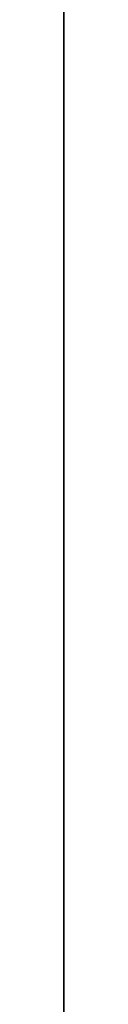
# Model space of a CAD drawing. Units: inches. Extents: x 2083 to 3317, y 1141 to 2115.
# Tile 44 of 256: x 2235.9598 to 2235.9598, y 1478.1958 to 1478.7355. Entities that reach past the tile are written whole.
import ezdxf

# ---------------------------------------------------------------- set-up
doc = ezdxf.new("R2010")
doc.units = ezdxf.units.IN
doc.layers.add('A-ANNO-DIMS', color=2, linetype='Continuous', lineweight=18)
doc.layers.add('A-WALL', color=7, linetype='Continuous', lineweight=35)
doc.layers.add('A-WALL-PATT', color=251, linetype='Continuous', lineweight=13, true_color=0x636466)
doc.styles.get("Standard").update_dxf_attribs({"font": 'arial.ttf'})
doc.dimstyles.new('ISO-25', dxfattribs={"dimtxt": 12, "dimasz": 12, "dimexe": 1.25, "dimexo": 0.625, "dimtad": 1, "dimlunit": 3, "dimtxsty": 'Standard', "dimcen": 2.5, "dimadec": 0, "dimazin": 0, "dimtfac": 1, "dimtmove": 0, "dimatfit": 3, "dimfxl": 1, "dimarcsym": 0})

# ---------------------------------------------------------------- blocks, each defined once
blk = doc.blocks.new('*D30')
at = {"layer": 'A-ANNO-DIMS', "color": 0, "lineweight": -2, "transparency": 16777216}
for p, q in [((2240.01786, 1445.27381), (2240.01786, 1448.04553)), ((2254.32933, 1445.27381), (2254.32933, 1448.04553)), ((2228.01786, 1446.79553), (2216.01786, 1446.79553)), ((2240.01786, 1446.79553), (2254.32933, 1446.79553)), ((2266.32933, 1446.79553), (2413.76487, 1446.79553))]:
    blk.add_line(p, q, dxfattribs=at)
at = {"layer": 'A-ANNO-DIMS', "color": 0, "transparency": 16777216}
for points in [[(2228.01786, 1448.79553), (2228.01786, 1444.79553), (2240.01786, 1446.79553)], [(2266.32933, 1448.79553), (2266.32933, 1444.79553), (2254.32933, 1446.79553)]]:
    blk.add_solid(points, dxfattribs=at)
at = {"layer": 'Defpoints', "color": 0, "transparency": 16777216}
for p in [(2254.32933, 1446.79553), (2240.01786, 1444.64881), (2254.32933, 1444.64881)]:
    blk.add_point(p, dxfattribs=at)
at = {"layer": 'A-ANNO-DIMS', "color": 0, "transparency": 16777216, "insert": (2346.0471, 1453.62517), "char_height": 12, "attachment_point": 5}
blk.add_mtext('WC 1\'-2 1/2" TYP.', dxfattribs=at)
blk = doc.blocks.new('*D31')
at = {"layer": 'A-ANNO-DIMS', "color": 0, "lineweight": -2, "transparency": 16777216}
for p, q in [((2237.87114, 1456.64881), (2237.87114, 1541.91518)), ((2239.39286, 1444.64881), (2236.62114, 1444.64881)), ((2237.87114, 1431.54754), (2237.87114, 1444.64881)), ((2239.39286, 1431.54754), (2236.62114, 1431.54754)), ((2237.87114, 1419.54754), (2237.87114, 1407.54754))]:
    blk.add_line(p, q, dxfattribs=at)
at = {"layer": 'A-ANNO-DIMS', "color": 0, "transparency": 16777216}
for points in [[(2235.87114, 1456.64881), (2239.87114, 1456.64881), (2237.87114, 1444.64881)], [(2235.87114, 1419.54754), (2239.87114, 1419.54754), (2237.87114, 1431.54754)]]:
    blk.add_solid(points, dxfattribs=at)
at = {"layer": 'Defpoints', "color": 0, "transparency": 16777216}
for p in [(2237.87114, 1444.64881), (2240.01786, 1444.64881), (2240.01786, 1431.54754)]:
    blk.add_point(p, dxfattribs=at)
at = {"layer": 'A-ANNO-DIMS', "color": 0, "transparency": 16777216, "insert": (2231.21749, 1505.28199), "char_height": 12, "attachment_point": 5, "rotation": 90}
blk.add_mtext('1\'-1" TYP.', dxfattribs=at)
blk = doc.blocks.new('*D45')
at = {"layer": 'A-ANNO-DIMS', "color": 0, "lineweight": -2, "transparency": 16777216}
for p, q in [((2235.95978, 1478.38636), (2235.95978, 1531.36136)), ((2418.95978, 1478.38636), (2418.95978, 1531.36136)), ((2247.95978, 1530.11136), (2406.95978, 1530.11136))]:
    blk.add_line(p, q, dxfattribs=at)
at = {"layer": 'A-ANNO-DIMS', "color": 0, "transparency": 16777216}
for points in [[(2247.95978, 1532.11136), (2247.95978, 1528.11136), (2235.95978, 1530.11136)], [(2406.95978, 1532.11136), (2406.95978, 1528.11136), (2418.95978, 1530.11136)]]:
    blk.add_solid(points, dxfattribs=at)
at = {"layer": 'Defpoints', "color": 0, "transparency": 16777216}
for p in [(2418.95978, 1530.11136), (2235.95978, 1477.76136), (2418.95978, 1477.76136)]:
    blk.add_point(p, dxfattribs=at)
at = {"layer": 'A-ANNO-DIMS', "color": 0, "transparency": 16777216, "insert": (2327.45978, 1536.86733), "char_height": 12, "attachment_point": 5}
blk.add_mtext('15\'-3"', dxfattribs=at)
blk = doc.blocks.new('*D62')
at = {"layer": 'A-ANNO-DIMS', "color": 0, "lineweight": -2, "transparency": 16777216}
for p, q in [((2235.95978, 1469.38636), (2235.95978, 1522.36136)), ((2379.95978, 1469.38636), (2379.95978, 1522.36136)), ((2247.95978, 1521.11136), (2367.95978, 1521.11136))]:
    blk.add_line(p, q, dxfattribs=at)
at = {"layer": 'A-ANNO-DIMS', "color": 0, "transparency": 16777216}
for points in [[(2247.95978, 1523.11136), (2247.95978, 1519.11136), (2235.95978, 1521.11136)], [(2367.95978, 1523.11136), (2367.95978, 1519.11136), (2379.95978, 1521.11136)]]:
    blk.add_solid(points, dxfattribs=at)
at = {"layer": 'Defpoints', "color": 0, "transparency": 16777216}
for p in [(2379.95978, 1521.11136), (2235.95978, 1468.76136), (2379.95978, 1468.76136)]:
    blk.add_point(p, dxfattribs=at)
at = {"layer": 'A-ANNO-DIMS', "color": 0, "transparency": 16777216, "insert": (2307.95978, 1527.86324), "char_height": 12, "attachment_point": 5}
blk.add_mtext('12\'-0"', dxfattribs=at)

msp = doc.modelspace()

# ---------------------------------------------------------------- hatches: boundary and pattern name
at = {"layer": 'A-WALL-PATT'}
h = msp.add_hatch(color=256, dxfattribs=at)
h.dxf.hatch_style = 1
h.paths.add_polyline_path([(3126.95978, 2020.76136), (2748.95978, 2020.76136), (2604.95978, 2020.76136), (2226.95978, 2020.76136), (2226.95978, 1702.76136), (2466.95978, 1702.76136), (2466.95978, 1582.76136), (2418.95978, 1582.76136), (2418.95978, 1477.76136), (2226.95978, 1477.76136), (2226.95978, 1263.26136), (2544.95978, 1263.26136), (2544.95978, 1411.76136), (2604.95978, 1411.76136), (2685.95978, 1411.76136), (2685.95978, 1420.76136), (2604.95978, 1420.76136), (2604.95978, 1573.76136), (2604.95978, 1702.76136), (2604.95978, 2011.76136), (2748.95978, 2011.76136), (2748.95978, 1702.76136), (2862.95978, 1702.76136), (2862.95978, 1621.76136), (2871.95978, 1621.76136), (2871.95978, 1702.76136), (2883.95978, 1702.76136), (2883.95978, 1706.93946, -0.026459), (2883.95978, 1711.76136), (2757.95978, 1711.76136), (2757.95978, 1807.76136), (2787.95978, 1807.76136), (2787.95978, 1812.26136), (2757.95978, 1812.26136), (2757.95978, 2011.76136), (2877.95978, 2011.76136), (2877.95978, 1812.26136), (2847.95978, 1812.26136), (2847.95978, 1807.76136), (2889.83574, 1807.76136), (2889.83574, 1812.26136), (2882.45978, 1812.26136), (2882.45978, 2011.76136), (3117.95978, 2011.76136), (3117.95978, 1812.26136), (2937.83574, 1812.26136), (2937.83574, 1807.76136), (2995.70978, 1807.76136), (2995.70978, 1796.11767), (3000.20978, 1796.11767), (3000.20978, 1807.76136), (3117.95978, 1807.76136), (3117.95978, 1711.76136), (3000.20978, 1711.76136), (3000.20978, 1760.11767), (2998.5727, 1760.11767, -0.020711), (2995.70978, 1760.11767), (2995.70978, 1711.76136), (2931.95978, 1711.76136), (2931.95978, 1702.76136), (3126.95978, 1702.76136)])
h.paths.add_polyline_path([(2471.45978, 2011.76136), (2471.45978, 1810.01136), (2462.71694, 1810.01136), (2462.71694, 1805.51136), (2505.95978, 1805.51136), (2505.95978, 1810.01136), (2475.95978, 1810.01136), (2475.95978, 2011.76136), (2595.95978, 2011.76136), (2595.95978, 1810.01136), (2565.95978, 1810.01136), (2565.95978, 1805.51136), (2595.95978, 1805.51136), (2595.95978, 1711.76136), (2235.95978, 1711.76136), (2235.95978, 1805.51136), (2353.70978, 1805.51136), (2353.70978, 1796.05416), (2358.20978, 1796.05416), (2358.20978, 1805.51136), (2414.71694, 1805.51136), (2414.71694, 1810.01136), (2235.95978, 1810.01136), (2235.95978, 2011.76136)], flags=16)
h.paths.add_polyline_path([(2270.20473, 1994.61001), (2270.20473, 1970.61001), (2246.20473, 1970.61001), (2246.20473, 1994.61001)], flags=0)
edge = h.paths.add_edge_path(flags=0)
edge.add_ellipse((2332.02739, 1899.79818), major_axis=(-3.04299, 3.04299), ratio=0.1682525, start_angle=-161.33217, end_angle=-156.30711, ccw=False)
edge.add_ellipse((2333.08204, 1898.74353), major_axis=(-1.05465, 1.05465), ratio=0.4535321, start_angle=-123.37102, end_angle=-94.15911)
edge = h.paths.add_edge_path(flags=0)
edge.add_ellipse((2332.02739, 1968.87629), major_axis=(3.04299, 3.04299), ratio=0.1682525, start_angle=18.66783, end_angle=23.69289)
edge.add_spline(control_points=[(2332.9256, 1970.6911), (2332.22677, 1970.3361), (2330.89371, 1969.65891), (2328.41308, 1970.93214), (2327.20393, 1967.74871), (2324.7096, 1969.95559), (2322.53282, 1967.01235), (2320.01285, 1971.29581), (2317.68031, 1968.15784), (2316.04053, 1967.10205), (2315.4269, 1966.8096)], knot_values=[0, 0, 0, 0, 2.267059, 4.324559, 6.685584, 8.878641, 11.121502, 14.300359, 17.755284, 19.732645, 19.732645, 19.732645, 19.732645], degree=3, periodic=0)
edge.add_ellipse((2332.02739, 1968.87629), major_axis=(3.04299, 3.04299), ratio=0.1682525, start_angle=18.66783, end_angle=23.69289, ccw=False)
edge.add_ellipse((2333.08204, 1969.93094), major_axis=(1.05465, 1.05465), ratio=0.4535321, start_angle=56.62898, end_angle=85.84089, ccw=False)
edge = h.paths.add_edge_path(flags=0)
edge.add_spline(control_points=[(2296.42829, 1967.98791), (2293.6278, 1965.33631), (2287.70362, 1959.72709), (2299.74386, 1949.9957), (2294.53259, 1935.66853), (2290.57323, 1920.60351), (2293.39412, 1909.97369), (2296.18541, 1904.96654)], knot_values=[0.099185, 0.099185, 0.099185, 0.099185, 0.345301, 0.619822, 0.982653, 1.386093, 1.810555, 1.810555, 1.810555, 1.810555], degree=3, periodic=0)
edge.add_spline(control_points=[(2296.18541, 1904.96654), (2297.38358, 1902.6193), (2298.00097, 1901.94931), (2298.55297, 1901.46815)], knot_values=[0.006246, 0.006246, 0.006246, 0.006246, 0.055476, 0.055476, 0.055476, 0.055476], degree=3, periodic=0)
edge.add_spline(control_points=[(2298.55297, 1901.46815), (2297.25861, 1900.92322), (2295.22529, 1900.23213), (2293.06023, 1900.61421), (2292.10142, 1900.78841), (2292.08958, 1900.79057)], knot_values=[0.312835, 0.312835, 0.312835, 0.312835, 0.40178, 0.474987, 0.475903, 0.475903, 0.475903, 0.475903], degree=3, periodic=0)
edge.add_arc((2292.79365, 1904.66411), 3.93701, 215.4209, 259.69818, ccw=False)
edge.add_spline(control_points=[(2289.58531, 1902.3823), (2289.47665, 1902.53509), (2289.36848, 1902.68804), (2289.26086, 1902.84117)], knot_values=[0.102872, 0.102872, 0.102872, 0.102872, 0.116896, 0.116896, 0.116896, 0.116896], degree=3, periodic=0)
edge.add_spline(control_points=[(2289.26086, 1902.84117), (2288.6866, 1902.55019), (2287.64005, 1902.0199), (2285.88134, 1901.87395), (2283.85297, 1901.50435), (2281.71999, 1899.71054), (2278.46699, 1899.49294), (2276.15714, 1901.8832), (2272.25895, 1899.80407), (2267.77761, 1901.84318), (2262.24388, 1900.18403), (2257.41493, 1901.78206), (2254.31837, 1900.72612), (2253.17828, 1900.33734)], knot_values=[0, 0, 0, 0, 1.907977, 3.477176, 5.261074, 7.972851, 11.680248, 13.717921, 16.939592, 22.789562, 27.502503, 33.595215, 37.145618, 37.145618, 37.145618, 37.145618], degree=3, periodic=0)
edge.add_line((2253.17828, 1900.33734), (2250.24424, 1902.84117))
edge.add_line((2250.24424, 1902.84117), (2250.24424, 1965.8333))
edge.add_line((2250.24424, 1965.8333), (2253.17828, 1968.33712))
edge.add_spline(control_points=[(2253.17828, 1968.33712), (2254.31837, 1967.94835), (2257.41493, 1966.89241), (2262.24388, 1968.49043), (2267.77761, 1966.83128), (2271.52673, 1968.53722), (2273.87591, 1967.82829), (2274.2067, 1967.72764)], knot_values=[0, 0, 0, 0, 0.09018, 0.244935, 0.364644, 0.513233, 0.537855, 0.537855, 0.537855, 0.537855], degree=3, periodic=0)
edge.add_arc((2274.35289, 1963.79335), 3.93701, 72.05113, 92.12795, ccw=False)
edge.add_arc((2281.29693, 1985.23), 18.5963, 252.051134, 288.565722)
edge.add_arc((2292.31672, 1956.02888), 12.64608, 71.026788, 113.778218, ccw=False)
edge = h.paths.add_edge_path(flags=0)
edge.add_spline(control_points=[(2274.89941, 1951.85619), (2275.06616, 1951.61659), (2275.23269, 1951.37659), (2275.39799, 1951.13585)], knot_values=[1.409916, 1.409916, 1.409916, 1.409916, 1.43159, 1.43159, 1.43159, 1.43159], degree=3, periodic=0)
edge.add_spline(control_points=[(2275.39799, 1951.13585), (2275.79211, 1950.56189), (2276.17923, 1949.98377), (2276.54555, 1949.3971)], knot_values=[1.358238, 1.358238, 1.358238, 1.358238, 1.409916, 1.409916, 1.409916, 1.409916], degree=3, periodic=0)
edge.add_line((2276.54555, 1949.3971), (2277.43729, 1947.86218))
edge.add_spline(control_points=[(2277.43729, 1947.86218), (2276.30383, 1945.67311), (2274.6397, 1942.42688), (2274.63161, 1938.0939), (2272.79912, 1930.85155), (2274.35643, 1943.89705), (2275.94768, 1947.92336), (2276.54555, 1949.3971)], knot_values=[0.005632, 0.005632, 0.005632, 0.005632, 0.186014, 0.266002, 0.357087, 0.59639, 0.739732, 0.739732, 0.739732, 0.739732], degree=3, periodic=0)
edge.add_spline(control_points=[(2276.54555, 1949.3971), (2276.17923, 1949.98377), (2275.79211, 1950.56189), (2275.39799, 1951.13585)], knot_values=[1.358238, 1.358238, 1.358238, 1.358238, 1.409916, 1.409916, 1.409916, 1.409916], degree=3, periodic=0)
edge.add_spline(control_points=[(2275.39799, 1951.13585), (2274.9425, 1950.08045), (2274.20776, 1948.02527), (2273.9346, 1944.85148), (2272.46853, 1937.62749), (2273.46622, 1945.69647), (2274.70062, 1951.05947), (2274.89941, 1951.85619)], knot_values=[0.104364, 0.104364, 0.104364, 0.104364, 0.189636, 0.269624, 0.36071, 0.600013, 0.644622, 0.644622, 0.644622, 0.644622], degree=3, periodic=0)
h.paths.add_polyline_path([(2269.16751, 1963.12757, -0.357527), (2268.17063, 1960.97637, -0.092561), (2268.17063, 1939.43632, -0.357527), (2269.16751, 1937.28512, -0.357527), (2267.01631, 1938.282, -0.164785), (2254.68558, 1938.282, -0.357527), (2252.53438, 1937.28512, -0.357527), (2253.53126, 1939.43632, -0.092561), (2253.53126, 1960.97637, -0.357527), (2252.53438, 1963.12757, -0.357527), (2254.68558, 1962.13069, -0.164785), (2267.01631, 1962.13069, -0.357527)], flags=0)
h.paths.add_polyline_path([(2248.87407, 1967.8018), (2248.87407, 1957.02771), (2249.45778, 1957.02771), (2249.45778, 1911.64676), (2248.87407, 1911.64676), (2248.87407, 1900.87267), (2246.51186, 1900.87267, 0.197327), (2244.14966, 1902.45687), (2244.14966, 1966.21759, 0.197327), (2246.51186, 1967.8018)], flags=0)
h.paths.add_polyline_path([(2269.16751, 1931.38934, -0.357527), (2268.17063, 1929.23814, -0.092561), (2268.17063, 1907.6981, -0.357527), (2269.16751, 1905.54689, -0.357527), (2267.01631, 1906.54377, -0.164785), (2254.68558, 1906.54377, -0.357527), (2252.53438, 1905.54689, -0.357527), (2253.53126, 1907.6981, -0.092561), (2253.53126, 1929.23814, -0.357527), (2252.53438, 1931.38934, -0.357527), (2254.68558, 1930.39246, -0.164785), (2267.01631, 1930.39246, -0.357527)], flags=0)
edge = h.paths.add_edge_path(flags=0)
edge.add_spline(control_points=[(2276.19686, 1906.7237), (2276.16814, 1909.02893), (2276.11405, 1913.37185), (2270.59842, 1924.92498), (2273.90517, 1919.01278), (2275.92171, 1916.26206), (2275.47457, 1912.40215), (2277.25787, 1910.38062), (2276.69604, 1908.22504), (2276.64622, 1906.81302), (2276.61782, 1906.00841)], knot_values=[0, 0, 0, 0, 8.61026, 16.221274, 18.843057, 23.804898, 27.440828, 29.356102, 31.203478, 33.650687, 33.650687, 33.650687, 33.650687], degree=3, periodic=0)
edge.add_spline(control_points=[(2276.61782, 1906.00841), (2276.62331, 1905.62414), (2276.49774, 1904.62866), (2275.44178, 1903.85473), (2274.93731, 1903.08045), (2274.85908, 1902.84117)], knot_values=[0.156488, 0.156488, 0.156488, 0.156488, 0.184398, 0.231376, 0.250598, 0.250598, 0.250598, 0.250598], degree=3, periodic=0)
edge.add_line((2274.85908, 1902.84117), (2276.50598, 1902.84117))
edge.add_spline(control_points=[(2276.50598, 1902.84117), (2276.78831, 1903.08494), (2277.66507, 1904.1252), (2278.24954, 1904.34074), (2277.65387, 1908.52739), (2278.15567, 1906.22781), (2278.10046, 1905.28595), (2278.84667, 1904.06901), (2277.85679, 1903.41495), (2277.87419, 1902.99105), (2277.90356, 1902.84117)], knot_values=[0.059574, 0.059574, 0.059574, 0.059574, 0.080753, 0.103741, 0.16972, 0.176036, 0.207137, 0.240474, 0.262341, 0.27366, 0.27366, 0.27366, 0.27366], degree=3, periodic=0)
edge.add_line((2277.90356, 1902.84117), (2280.02983, 1902.84117))
edge.add_spline(control_points=[(2280.02983, 1902.84117), (2279.88822, 1903.0884), (2279.49926, 1903.98155), (2280.15228, 1905.93935), (2278.10362, 1909.65776), (2279.76239, 1907.18529), (2280.3279, 1904.87486), (2280.48511, 1903.48959), (2281.46327, 1903.24943), (2281.75834, 1902.9365), (2281.83404, 1902.84117)], knot_values=[0.013856, 0.013856, 0.013856, 0.013856, 0.034874, 0.088867, 0.107879, 0.126738, 0.158714, 0.193757, 0.217487, 0.226722, 0.226722, 0.226722, 0.226722], degree=3, periodic=0)
edge.add_spline(control_points=[(2281.83404, 1902.84117), (2281.78753, 1902.8267), (2281.64702, 1902.78299), (2281.39553, 1902.85949), (2281.08808, 1902.98524), (2280.72068, 1903.0609), (2280.33345, 1903.02573), (2280.12477, 1902.89888), (2280.02983, 1902.84117)], knot_values=[0, 0, 0, 0, 0.14413, 0.435517, 0.749276, 1.153046, 1.548371, 1.878348, 1.878348, 1.878348, 1.878348], degree=3, periodic=0)
edge.add_line((2280.02983, 1902.84117), (2277.90356, 1902.84117))
edge.add_spline(control_points=[(2277.90356, 1902.84117), (2277.89286, 1902.79586), (2277.8654, 1902.67964), (2277.60748, 1902.68748), (2277.27405, 1902.8007), (2276.83792, 1902.61977), (2276.58381, 1902.78926), (2276.50598, 1902.84117)], knot_values=[0, 0, 0, 0, 0.127189, 0.326199, 0.628009, 1.24357, 1.515331, 1.515331, 1.515331, 1.515331], degree=3, periodic=0)
edge.add_line((2276.50598, 1902.84117), (2274.85908, 1902.84117))
edge.add_spline(control_points=[(2274.85908, 1902.84117), (2274.81444, 1902.89859), (2274.72513, 1903.01345), (2274.49348, 1903.11897), (2274.24429, 1902.96054), (2273.93712, 1903.18494), (2273.61404, 1902.98314), (2273.40832, 1902.88304), (2273.32225, 1902.84117)], knot_values=[0, 0, 0, 0, 0.21843, 0.436957, 0.687977, 0.990379, 1.398396, 1.69185, 1.69185, 1.69185, 1.69185], degree=3, periodic=0)
edge.add_spline(control_points=[(2273.32225, 1902.84117), (2273.61674, 1903.44569), (2274.274, 1904.53825), (2276.02724, 1904.5737), (2276.20696, 1906.58364), (2276.19686, 1906.7237)], knot_values=[0.012227, 0.012227, 0.012227, 0.012227, 0.059472, 0.106218, 0.134458, 0.134458, 0.134458, 0.134458], degree=3, periodic=0)
h.paths.add_polyline_path([(2270.77605, 1897.78983), (2270.77605, 1873.78983), (2246.77605, 1873.78983), (2246.77605, 1897.78983)], flags=0)
h.paths.add_polyline_path([(2353.70978, 1760.00506), (2353.70978, 1760.05416), (2358.20978, 1760.05416, -0.033729)], flags=0)
h.paths.add_polyline_path([(2321.81912, 1737.52919), (2341.99533, 1737.52919, -0.414214), (2343.20327, 1736.32124), (2343.20327, 1721.0206, -0.414214), (2341.99533, 1719.81265), (2321.81912, 1719.81265, -0.414214), (2320.61117, 1721.0206), (2320.61117, 1736.32124, -0.414214)], flags=0)
h.paths.add_polyline_path([(2324.23501, 1736.32124), (2339.57944, 1736.32124, -0.414214), (2341.99533, 1733.90535), (2341.99533, 1725.44973, -0.414214), (2339.57944, 1723.03384), (2333.68059, 1723.03384), (2333.84532, 1722.04547, -0.870646), (2335.4254, 1721.82589, -0.767327), (2333.92269, 1721.42324), (2331.29102, 1721.42324, -0.767327), (2329.78832, 1721.82589, -0.870646), (2331.3684, 1722.04547), (2331.53313, 1723.03384), (2324.23501, 1723.03384, -0.414214), (2321.81912, 1725.44973), (2321.81912, 1733.90535, -0.414214)], flags=0)
h.paths.add_polyline_path([(2570.48379, 1928.61544), (2589.68379, 1928.61544), (2590.16883, 1928.61544), (2590.16883, 1904.9934), (2570.48379, 1904.9934)], flags=0)
h.paths.add_polyline_path([(2574.44732, 1927.26382, -1), (2572.82884, 1927.26382, -1)], flags=0)
h.paths.add_polyline_path([(2573.08987, 1926.94088), (2573.92503, 1927.77604), (2574.14774, 1927.55333), (2573.31258, 1926.71817)], flags=0)
h.paths.add_polyline_path([(2578.77906, 1919.72962, -1), (2571.59166, 1919.72962, -1)], flags=0)
h.paths.add_polyline_path([(2578.38536, 1919.72962, -1), (2571.98536, 1919.72962, -1)], flags=0)
h.paths.add_polyline_path([(2331.59576, 1729.47622, -1), (2333.61795, 1729.47622, -1)], flags=0)
h.paths.add_polyline_path([(2578.03423, 1927.26382, -1), (2576.41574, 1927.26382, -1)], flags=0)
h.paths.add_polyline_path([(2576.68885, 1927.53109), (2576.91156, 1927.7538), (2577.74673, 1926.91863), (2577.52402, 1926.69592)], flags=0)
h.paths.add_polyline_path([(2578.13906, 1909.85954, -1), (2572.23166, 1909.85954, -1)], flags=0)
h.paths.add_polyline_path([(2577.74536, 1909.85954, -1), (2572.62536, 1909.85954, -1)], flags=0)
h.paths.add_polyline_path([(2583.79772, 1927.26382, -1), (2582.17923, 1927.26382, -1)], flags=0)
h.paths.add_polyline_path([(2582.71865, 1927.7538), (2583.55381, 1926.91863), (2583.3311, 1926.69592), (2582.49594, 1927.53109)], flags=0)
h.paths.add_polyline_path([(2582.49594, 1927.53109), (2582.71865, 1927.7538), (2583.55381, 1926.91863), (2583.3311, 1926.69592)], flags=0)
h.paths.add_polyline_path([(2587.73906, 1920.52962, -1), (2581.83166, 1920.52962, -1)], flags=0)
h.paths.add_polyline_path([(2587.34536, 1920.52962, -1), (2582.22536, 1920.52962, -1)], flags=0)
h.paths.add_polyline_path([(2587.38462, 1927.26382, -1), (2585.76613, 1927.26382, -1)], flags=0)
h.paths.add_polyline_path([(2586.08199, 1926.98025), (2586.91716, 1927.81541), (2587.13987, 1927.5927), (2586.3047, 1926.75754)], flags=0)
h.paths.add_polyline_path([(2588.37906, 1910.65954, -1), (2581.19166, 1910.65954, -1)], flags=0)
h.paths.add_polyline_path([(2587.98536, 1910.65954, -1), (2581.58536, 1910.65954, -1)], flags=0)
h.paths.add_polyline_path([(2417.16773, 1729.4779), (2437.34394, 1729.4779, -0.414214), (2438.55188, 1728.26995), (2438.55188, 1712.96931, -0.414214), (2437.34394, 1711.76136), (2417.16773, 1711.76136, -0.414214), (2415.95978, 1712.96931), (2415.95978, 1728.26995, -0.414214)], flags=0)
h.paths.add_polyline_path([(2419.58362, 1728.26995), (2434.92805, 1728.26995, -0.414214), (2437.34394, 1725.85406), (2437.34394, 1717.39844, -0.414214), (2434.92805, 1714.98255), (2429.0292, 1714.98255), (2429.19393, 1713.99418, -0.870646), (2430.77401, 1713.7746, -0.767327), (2429.2713, 1713.37195), (2426.63963, 1713.37195, -0.767327), (2425.13693, 1713.7746, -0.870646), (2426.71701, 1713.99418), (2426.88174, 1714.98255), (2419.58362, 1714.98255, -0.414214), (2417.16773, 1717.39844), (2417.16773, 1725.85406, -0.414214)], flags=0)
h.paths.add_polyline_path([(2419.58362, 1728.26995), (2434.92805, 1728.26995, -0.414214), (2437.34394, 1725.85406), (2437.34394, 1717.39844, -0.414214), (2434.92805, 1714.98255), (2429.0292, 1714.98255), (2428.35812, 1719.00903), (2427.55282, 1719.00903), (2426.88174, 1714.98255), (2419.58362, 1714.98255, -0.414214), (2417.16773, 1717.39844), (2417.16773, 1725.85406, -0.414214)], flags=0)
h.paths.add_polyline_path([(2426.94437, 1721.42492, -1), (2428.96656, 1721.42492, -1)], flags=0)
h.paths.add_polyline_path([(2475.95978, 1702.76136), (2595.95978, 1702.76136), (2595.95978, 1582.76136), (2475.95978, 1582.76136)], flags=16)
h.paths.add_polyline_path([(2427.95978, 1573.76136), (2595.95978, 1573.76136), (2595.95978, 1468.76136), (2595.95978, 1420.76136), (2384.45978, 1420.76136), (2384.45978, 1468.76136), (2427.95978, 1468.76136)], flags=16)
h.paths.add_polyline_path([(2379.95978, 1468.76136), (2379.95978, 1420.76136), (2235.95978, 1420.76136), (2235.95978, 1468.76136)], flags=16)
h.paths.add_polyline_path([(2317.816, 1466.69577), (2337.9922, 1466.69577, -0.414214), (2339.20015, 1465.48782), (2339.20015, 1450.18718, -0.414214), (2337.9922, 1448.97923), (2317.816, 1448.97923, -0.414214), (2316.60805, 1450.18718), (2316.60805, 1465.48782, -0.414214)], flags=0)
h.paths.add_polyline_path([(2320.23189, 1465.48782), (2335.57631, 1465.48782, -0.414214), (2337.9922, 1463.07193), (2337.9922, 1454.61631, -0.414214), (2335.57631, 1452.20042), (2329.67747, 1452.20042), (2329.84219, 1451.21205, -0.870646), (2331.42228, 1450.99247, -0.767327), (2329.91957, 1450.58983), (2327.2879, 1450.58983, -0.767327), (2325.7852, 1450.99247, -0.870646), (2327.36528, 1451.21205), (2327.53001, 1452.20042), (2320.23189, 1452.20042, -0.414214), (2317.816, 1454.61631), (2317.816, 1463.07193, -0.414214)], flags=0)
h.paths.add_polyline_path([(2320.23189, 1465.48782), (2335.57631, 1465.48782, -0.414214), (2337.9922, 1463.07193), (2337.9922, 1454.61631, -0.414214), (2335.57631, 1452.20042), (2329.67747, 1452.20042), (2329.00638, 1456.22691), (2328.20109, 1456.22691), (2327.53001, 1452.20042), (2320.23189, 1452.20042, -0.414214), (2317.816, 1454.61631), (2317.816, 1463.07193, -0.414214)], flags=0)
h.paths.add_polyline_path([(2327.59264, 1458.6428, -1), (2329.61483, 1458.6428, -1)], flags=0)
h.paths.add_polyline_path([(2244.41174, 1433.34045), (2241.92094, 1433.34045, -0.414214), (2240.01786, 1435.24354), (2240.01786, 1440.95281, -0.414211), (2241.92093, 1442.8559), (2244.41174, 1442.8559, -1.976472)], flags=0)
h.paths.add_polyline_path([(2245.35689, 1434.39754, -0.414214), (2245.35689, 1441.79881, -2.144098)], flags=0)
h.paths.add_polyline_path([(2535.95978, 1416.26136), (2535.95978, 1272.26136), (2235.95978, 1272.26136), (2235.95978, 1416.26136)], flags=16)
h.paths.add_polyline_path([(2260.11956, 1384.29284), (2260.11956, 1362.03865), (2237.86537, 1362.03865), (2237.86537, 1384.29284)], flags=0)
edge = h.paths.add_edge_path(flags=0)
edge.add_line((2318.25185, 1362.0933), (2318.1458, 1362.00097))
edge.add_ellipse((2317.44512, 1360.43104), major_axis=(2.82164, 2.82164), ratio=0.1682525, start_angle=18.66783, end_angle=20.94813, ccw=False)
edge.add_ellipse((2318.42305, 1361.40897), major_axis=(0.97793, 0.97793), ratio=0.4535321, start_angle=56.62898, end_angle=70.2262, ccw=False)
edge = h.paths.add_edge_path(flags=0)
edge.add_line((2319.10737, 1295.57108), (2319.01504, 1295.67713))
edge.add_ellipse((2317.44512, 1296.37781), major_axis=(-2.82164, 2.82164), ratio=0.1682525, start_angle=-161.33217, end_angle=-159.05187, ccw=False)
edge.add_ellipse((2318.42305, 1295.39988), major_axis=(-0.97793, 0.97793), ratio=0.4535321, start_angle=-123.37102, end_angle=-109.7738)
edge = h.paths.add_edge_path(flags=0)
edge.add_spline(control_points=[(2284.21035, 1301.17022), (2284.58069, 1300.44472), (2284.89119, 1299.89202), (2285.15955, 1299.46102)], knot_values=[0.039066, 0.039066, 0.039066, 0.039066, 0.055476, 0.055476, 0.055476, 0.055476], degree=3, periodic=0)
edge.add_line((2285.15955, 1299.46102), (2284.21035, 1301.17022))
edge = h.paths.add_edge_path(flags=0)
edge.add_line((2280.41246, 1297.29801), (2283.36999, 1297.03612))
edge.add_line((2283.36999, 1297.03612), (2286.40569, 1297.92631))
edge.add_spline(control_points=[(2286.40569, 1297.92631), (2285.30549, 1297.46312), (2284.34478, 1297.12915), (2283.36999, 1297.03612)], knot_values=[0.394369, 0.394369, 0.394369, 0.394369, 0.475903, 0.475903, 0.475903, 0.475903], degree=3, periodic=0)
edge.add_spline(control_points=[(2283.36999, 1297.03612), (2283.28139, 1297.02767), (2282.31629, 1296.95734), (2281.3125, 1297.13448), (2280.42344, 1297.29602), (2280.41246, 1297.29801)], knot_values=[0.312835, 0.312835, 0.312835, 0.312835, 0.320246, 0.393453, 0.394369, 0.394369, 0.394369, 0.394369], degree=3, periodic=0)
edge = h.paths.add_edge_path(flags=0)
edge.add_line((2284.43556, 1359.60729), (2280.44629, 1355.32805))
edge.add_line((2280.44629, 1355.32805), (2279.57999, 1351.01775))
edge.add_line((2279.57999, 1351.01775), (2282.41297, 1346.58043))
edge.add_spline(control_points=[(2282.41297, 1346.58043), (2283.15333, 1345.58924), (2284.2529, 1344.0289), (2284.80104, 1342.38717), (2284.93516, 1341.80554)], knot_values=[1.240098, 1.240098, 1.240098, 1.240098, 1.332892, 1.382712, 1.382712, 1.382712, 1.382712], degree=3, periodic=0)
edge.add_spline(control_points=[(2284.93516, 1341.80554), (2285.31911, 1340.1406), (2285.23303, 1338.4092), (2284.90994, 1336.65412)], knot_values=[1.097484, 1.097484, 1.097484, 1.097484, 1.240098, 1.240098, 1.240098, 1.240098], degree=3, periodic=0)
edge.add_spline(control_points=[(2284.90994, 1336.65412), (2284.58685, 1334.89904), (2284.02675, 1333.12027), (2283.46264, 1331.36058)], knot_values=[0.95487, 0.95487, 0.95487, 0.95487, 1.097484, 1.097484, 1.097484, 1.097484], degree=3, periodic=0)
edge.add_line((2283.46264, 1331.36058), (2281.89038, 1326.15336))
edge.add_line((2281.89038, 1326.15336), (2280.75626, 1321.05609))
edge.add_line((2280.75626, 1321.05609), (2280.2992, 1316.00198))
edge.add_line((2280.2992, 1316.00198), (2280.71593, 1310.95007))
edge.add_line((2280.71593, 1310.95007), (2282.02809, 1305.97214))
edge.add_line((2282.02809, 1305.97214), (2284.21035, 1301.17022))
edge.add_spline(control_points=[(2284.21035, 1301.17022), (2283.34073, 1302.73019), (2282.6119, 1304.33649), (2282.02809, 1305.97214)], knot_values=[0.099185, 0.099185, 0.099185, 0.099185, 0.241799, 0.241799, 0.241799, 0.241799], degree=3, periodic=0)
edge.add_spline(control_points=[(2282.02809, 1305.97214), (2281.44428, 1307.60778), (2281.00549, 1309.27276), (2280.71593, 1310.95007)], knot_values=[0.241799, 0.241799, 0.241799, 0.241799, 0.384413, 0.384413, 0.384413, 0.384413], degree=3, periodic=0)
edge.add_spline(control_points=[(2280.71593, 1310.95007), (2280.43324, 1312.58761), (2280.28939, 1314.27696), (2280.29889, 1315.96203), (2280.2992, 1316.00198)], knot_values=[0.384413, 0.384413, 0.384413, 0.384413, 0.523647, 0.527028, 0.527028, 0.527028, 0.527028], degree=3, periodic=0)
edge.add_spline(control_points=[(2280.2992, 1316.00198), (2280.31233, 1317.68696), (2280.47787, 1319.36793), (2280.75626, 1321.05609)], knot_values=[0.527028, 0.527028, 0.527028, 0.527028, 0.669642, 0.669642, 0.669642, 0.669642], degree=3, periodic=0)
edge.add_spline(control_points=[(2280.75626, 1321.05609), (2281.03465, 1322.74425), (2281.42588, 1324.43961), (2281.89038, 1326.15336)], knot_values=[0.669642, 0.669642, 0.669642, 0.669642, 0.812256, 0.812256, 0.812256, 0.812256], degree=3, periodic=0)
edge.add_spline(control_points=[(2281.89038, 1326.15336), (2282.26438, 1327.53325), (2282.78787, 1329.26181), (2283.35275, 1331.01778), (2283.46264, 1331.36058)], knot_values=[0.812256, 0.812256, 0.812256, 0.812256, 0.927087, 0.95487, 0.95487, 0.95487, 0.95487], degree=3, periodic=0)
edge.add_line((2283.46264, 1331.36058), (2284.90994, 1336.65412))
edge.add_line((2284.90994, 1336.65412), (2284.93516, 1341.80554))
edge.add_line((2284.93516, 1341.80554), (2282.41297, 1346.58043))
edge.add_spline(control_points=[(2282.41297, 1346.58043), (2281.27513, 1348.10379), (2280.07845, 1349.57032), (2279.57999, 1351.01775)], knot_values=[1.382712, 1.382712, 1.382712, 1.382712, 1.525326, 1.525326, 1.525326, 1.525326], degree=3, periodic=0)
edge.add_spline(control_points=[(2279.57999, 1351.01775), (2279.44328, 1351.41472), (2279.13631, 1352.85692), (2279.73519, 1354.29039), (2280.44629, 1355.32805)], knot_values=[1.525326, 1.525326, 1.525326, 1.525326, 1.564439, 1.667941, 1.667941, 1.667941, 1.667941], degree=3, periodic=0)
edge.add_spline(control_points=[(2280.44629, 1355.32805), (2281.42611, 1356.75784), (2282.93084, 1358.18256), (2284.43556, 1359.60729)], knot_values=[1.667941, 1.667941, 1.667941, 1.667941, 1.810555, 1.810555, 1.810555, 1.810555], degree=3, periodic=0)
edge.add_arc((2280.62307, 1348.51818), 11.72618, 71.026788, 113.778218)
edge.add_arc((2270.40489, 1375.59516), 17.24357, 252.051134, 288.565722, ccw=False)
edge.add_arc((2263.96597, 1355.71785), 3.65062, 72.05113, 92.12795)
edge.add_arc((2263.96597, 1355.71785), 3.65062, 92.12795, 177.98513)
edge.add_spline(control_points=[(2260.3176, 1355.8462), (2260.26042, 1354.22067), (2260.55128, 1350.18655), (2262.99934, 1346.76625), (2264.47274, 1344.64902)], knot_values=[1.43159, 1.43159, 1.43159, 1.43159, 1.564144, 1.770695, 1.770695, 1.770695, 1.770695], degree=3, periodic=0)
edge.add_line((2264.47274, 1344.64902), (2264.93559, 1343.98253))
edge.add_spline(control_points=[(2263.80104, 1340.24811), (2263.84324, 1340.51409), (2264.06724, 1341.75647), (2264.51269, 1343.00245), (2264.93505, 1343.98108)], knot_values=[0.53657, 0.53657, 0.53657, 0.53657, 0.559349, 0.644622, 0.644622, 0.644622, 0.644622], degree=3, periodic=0)
edge.add_spline(control_points=[(2264.93505, 1343.98108), (2265.11777, 1343.71497), (2265.29888, 1343.44791), (2265.47676, 1343.17936)], knot_values=[1.384077, 1.384077, 1.384077, 1.384077, 1.409916, 1.409916, 1.409916, 1.409916], degree=3, periodic=0)
edge.add_spline(control_points=[(2265.47676, 1343.17936), (2265.65464, 1342.91082), (2265.8293, 1342.64081), (2265.99913, 1342.36881)], knot_values=[1.358238, 1.358238, 1.358238, 1.358238, 1.384077, 1.384077, 1.384077, 1.384077], degree=3, periodic=0)
edge.add_line((2265.99913, 1342.36881), (2266.82601, 1340.94555))
edge.add_spline(control_points=[(2266.82601, 1340.94555), (2268.8944, 1337.08969), (2271.39817, 1325.843), (2270.51616, 1310.56856), (2275.91938, 1301.86061), (2277.78951, 1299.19945)], knot_values=[0.116896, 0.116896, 0.116896, 0.116896, 0.472987, 1.050969, 1.313793, 1.313793, 1.313793, 1.313793], degree=3, periodic=0)
edge.add_spline(control_points=[(2277.78951, 1299.19945), (2277.83941, 1299.12845), (2277.88943, 1299.0575), (2277.93957, 1298.98658)], knot_values=[0.109884, 0.109884, 0.109884, 0.109884, 0.116896, 0.116896, 0.116896, 0.116896], degree=3, periodic=0)
edge.add_line((2277.93957, 1298.98658), (2277.78885, 1299.19911))
edge.add_spline(control_points=[(2277.78885, 1299.19911), (2277.25658, 1298.92941), (2276.28635, 1298.4379), (2275.03935, 1298.33442), (2274.38333, 1298.2389), (2274.21525, 1298.20934)], knot_values=[33.12187, 33.12187, 33.12187, 33.12187, 35.029056, 36.598255, 37.144827, 37.144827, 37.144827, 37.144827], degree=3, periodic=0)
edge.add_line((2274.21525, 1298.20934), (2273.07315, 1297.89296))
edge.add_spline(control_points=[(2273.07315, 1297.89296), (2272.32294, 1297.57978), (2271.03915, 1296.51051), (2269.24839, 1296.22606), (2268.4231, 1296.37465)], knot_values=[26.532584, 26.532584, 26.532584, 26.532584, 29.198919, 31.839101, 31.839101, 31.839101, 31.839101], degree=3, periodic=0)
edge.add_line((2268.4231, 1296.37465), (2263.8785, 1297.45753))
edge.add_spline(control_points=[(2263.8785, 1297.45753), (2263.55608, 1297.35943), (2261.86031, 1296.83869), (2260.23878, 1297.28241), (2258.93345, 1297.51646)], knot_values=[15.919551, 15.919551, 15.919551, 15.919551, 16.939592, 21.226067, 21.226067, 21.226067, 21.226067], degree=3, periodic=0)
edge.add_line((2258.93345, 1297.51646), (2254.05523, 1297.32901))
edge.add_spline(control_points=[(2254.05523, 1297.32901), (2253.75553, 1297.29582), (2252.11368, 1297.16517), (2250.46187, 1297.54422), (2249.12969, 1297.66788)], knot_values=[5.306517, 5.306517, 5.306517, 5.306517, 6.276435, 10.613034, 10.613034, 10.613034, 10.613034], degree=3, periodic=0)
edge.add_line((2249.12969, 1297.66788), (2244.33165, 1296.87776))
edge.add_line((2244.33165, 1296.87776), (2241.61103, 1299.19945))
edge.add_line((2241.61103, 1299.19945), (2241.61103, 1357.6094))
edge.add_line((2241.61103, 1357.6094), (2244.33165, 1359.9311))
edge.add_line((2244.33165, 1359.9311), (2252.72882, 1359.54269))
edge.add_spline(control_points=[(2252.72882, 1359.54269), (2252.87094, 1359.54644), (2253.30574, 1359.54817), (2253.73984, 1359.51427), (2254.03174, 1359.48243)], knot_values=[0.233291, 0.233291, 0.233291, 0.233291, 0.244935, 0.268927, 0.268927, 0.268927, 0.268927], degree=3, periodic=0)
edge.add_line((2254.03174, 1359.48243), (2259.58719, 1359.41639))
edge.add_spline(control_points=[(2259.58719, 1359.41639), (2260.67707, 1359.6285), (2262.0732, 1359.897), (2263.52369, 1359.45928), (2263.83042, 1359.36595)], knot_values=[0.422516, 0.422516, 0.422516, 0.422516, 0.513233, 0.537855, 0.537855, 0.537855, 0.537855], degree=3, periodic=0)
edge.add_arc((2263.96597, 1355.71785), 3.65062, 72.05113, 92.12795, ccw=False)
edge.add_arc((2270.40489, 1375.59516), 17.24357, 252.051134, 288.565722)
edge.add_arc((2280.62307, 1348.51818), 11.72618, 71.026788, 113.778218, ccw=False)
h.paths.add_polyline_path([(2240.34053, 1359.43471), (2240.34053, 1349.44435), (2240.88178, 1349.44435), (2240.88178, 1307.3645), (2240.34053, 1307.3645), (2240.34053, 1297.37414), (2238.15016, 1297.37414, 0.197327), (2235.95978, 1298.84311), (2235.95978, 1357.96575, 0.197327), (2238.15016, 1359.43471)], flags=0)
h.paths.add_polyline_path([(2259.15779, 1355.1005, -0.357527), (2258.23342, 1353.10578, -0.092561), (2258.23342, 1333.1326, -0.357527), (2259.15779, 1331.13788, -0.357527), (2257.16307, 1332.06225, -0.164785), (2245.7293, 1332.06225, -0.357527), (2243.73458, 1331.13788, -0.357527), (2244.65895, 1333.1326, -0.092561), (2244.65895, 1353.10578, -0.357527), (2243.73458, 1355.1005, -0.357527), (2245.7293, 1354.17613, -0.164785), (2257.16307, 1354.17613, -0.357527)], flags=0)
edge = h.paths.add_edge_path(flags=0)
edge.add_line((2265.99913, 1342.36881), (2266.82601, 1340.94555))
edge.add_line((2266.82601, 1340.94555), (2265.30756, 1337.81407))
edge.add_line((2265.30756, 1337.81407), (2264.35823, 1334.65294))
edge.add_line((2264.35823, 1334.65294), (2264.26201, 1333.7997))
edge.add_spline(control_points=[(2264.26201, 1333.7997), (2264.20836, 1333.18705), (2264.16206, 1332.36553), (2264.00714, 1331.41393), (2263.96905, 1331.20183)], knot_values=[0.464444, 0.464444, 0.464444, 0.464444, 0.516691, 0.531608, 0.531608, 0.531608, 0.531608], degree=3, periodic=0)
edge.add_spline(control_points=[(2263.96905, 1331.20183), (2263.77453, 1330.11887), (2263.42437, 1328.79084), (2263.25742, 1328.53065), (2263.23403, 1328.51461)], knot_values=[0.372682, 0.372682, 0.372682, 0.372682, 0.44885, 0.464444, 0.464444, 0.464444, 0.464444], degree=3, periodic=0)
edge.add_spline(control_points=[(2263.23403, 1328.51461), (2263.09638, 1328.42023), (2263.13117, 1329.30148), (2263.27495, 1330.61575)], knot_values=[0.280919, 0.280919, 0.280919, 0.280919, 0.372682, 0.372682, 0.372682, 0.372682], degree=3, periodic=0)
edge.add_spline(control_points=[(2263.27495, 1330.61575), (2263.41874, 1331.93002), (2263.67152, 1333.67732), (2263.96985, 1335.31503)], knot_values=[0.189157, 0.189157, 0.189157, 0.189157, 0.280919, 0.280919, 0.280919, 0.280919], degree=3, periodic=0)
edge.add_spline(control_points=[(2263.96985, 1335.31503), (2264.1005, 1336.03219), (2264.41878, 1337.62191), (2264.75485, 1338.86443), (2264.94742, 1339.49112)], knot_values=[0.097394, 0.097394, 0.097394, 0.097394, 0.137578, 0.189157, 0.189157, 0.189157, 0.189157], degree=3, periodic=0)
edge.add_spline(control_points=[(2264.94742, 1339.49112), (2265.29002, 1340.60605), (2265.64424, 1341.494), (2265.99913, 1342.36881)], knot_values=[0.005632, 0.005632, 0.005632, 0.005632, 0.097394, 0.097394, 0.097394, 0.097394], degree=3, periodic=0)
h.paths.add_polyline_path([(2259.15779, 1325.67097, -0.357527), (2258.23342, 1323.67625, -0.092561), (2258.23342, 1303.70307, -0.357527), (2259.15779, 1301.70835, -0.357527), (2257.16307, 1302.63272, -0.164785), (2245.7293, 1302.63272, -0.357527), (2243.73458, 1301.70835, -0.357527), (2244.65895, 1303.70307, -0.092561), (2244.65895, 1323.67625, -0.357527), (2243.73458, 1325.67097, -0.357527), (2245.7293, 1324.74661, -0.164785), (2257.16307, 1324.74661, -0.357527)], flags=0)
edge = h.paths.add_edge_path(flags=0)
edge.add_spline(control_points=[(2261.70894, 1317.31142), (2261.67948, 1317.41758), (2261.76186, 1317.38853), (2262.49074, 1316.08987), (2262.96218, 1315.3009)], knot_values=[14.955861, 14.955861, 14.955861, 14.955861, 16.221274, 18.694826, 18.694826, 18.694826, 18.694826], degree=3, periodic=0)
edge.add_spline(control_points=[(2262.96218, 1315.3009), (2262.99044, 1315.25362), (2263.7021, 1314.06738), (2264.34898, 1313.12715), (2264.73005, 1312.16415)], knot_values=[18.694826, 18.694826, 18.694826, 18.694826, 18.843057, 22.433791, 22.433791, 22.433791, 22.433791], degree=3, periodic=0)
edge.add_spline(control_points=[(2264.73005, 1312.16415), (2264.87556, 1311.79644), (2265.17687, 1310.76981), (2265.14307, 1309.55926), (2265.24774, 1308.82419)], knot_values=[22.433791, 22.433791, 22.433791, 22.433791, 23.804898, 26.172756, 26.172756, 26.172756, 26.172756], degree=3, periodic=0)
edge.add_line((2265.24774, 1308.82419), (2265.85077, 1307.17189))
edge.add_spline(control_points=[(2265.85077, 1307.17189), (2266.06502, 1306.82168), (2266.38439, 1306.33225), (2266.4244, 1305.78055), (2266.42037, 1305.61122)], knot_values=[28.062562, 28.062562, 28.062562, 28.062562, 29.356102, 29.911721, 29.911721, 29.911721, 29.911721], degree=3, periodic=0)
edge.add_spline(control_points=[(2266.42037, 1305.61122), (2266.41612, 1305.43259), (2266.394, 1305.25), (2266.36478, 1305.06586)], knot_values=[29.911721, 29.911721, 29.911721, 29.911721, 30.497837, 30.497837, 30.497837, 30.497837], degree=3, periodic=0)
edge.add_line((2266.36478, 1305.06586), (2266.06615, 1302.1363))
edge.add_spline(control_points=[(2266.06615, 1302.1363), (2266.07124, 1301.77998), (2265.99808, 1301.19998), (2265.66327, 1300.75896), (2265.50891, 1300.58588)], knot_values=[0.156488, 0.156488, 0.156488, 0.156488, 0.184398, 0.203543, 0.203543, 0.203543, 0.203543], degree=3, periodic=0)
edge.add_line((2265.50891, 1300.58588), (2264.43534, 1299.19945))
edge.add_line((2264.43534, 1299.19945), (2265.96244, 1299.19945))
edge.add_line((2265.96244, 1299.19945), (2267.33599, 1301.17528))
edge.add_line((2267.33599, 1301.17528), (2267.31167, 1301.98624))
edge.add_spline(control_points=[(2267.31167, 1301.98624), (2267.26111, 1302.8624), (2267.16021, 1303.73713), (2267.27149, 1303.3259)], knot_values=[0.126229, 0.126229, 0.126229, 0.126229, 0.166617, 0.166617, 0.166617, 0.166617], degree=3, periodic=0)
edge.add_spline(control_points=[(2267.27149, 1303.3259), (2267.28003, 1303.2943), (2267.30979, 1303.17537), (2267.37345, 1302.88361), (2267.40612, 1302.68283), (2267.41793, 1302.60103)], knot_values=[0.166617, 0.166617, 0.166617, 0.166617, 0.16972, 0.176036, 0.180765, 0.180765, 0.180765, 0.180765], degree=3, periodic=0)
edge.add_spline(control_points=[(2267.74389, 1300.9875), (2267.68758, 1301.15094), (2267.48052, 1301.65666), (2267.48375, 1302.14479), (2267.41793, 1302.60103)], knot_values=[0.180765, 0.180765, 0.180765, 0.180765, 0.193767, 0.220139, 0.220139, 0.220139, 0.220139], degree=3, periodic=0)
edge.add_line((2267.41793, 1302.60103), (2267.74389, 1300.9875))
edge.add_spline(control_points=[(2267.74389, 1300.9875), (2267.83196, 1300.73188), (2267.93202, 1300.3099), (2267.55484, 1299.97452), (2267.42937, 1299.82921)], knot_values=[0.220139, 0.220139, 0.220139, 0.220139, 0.240474, 0.25489, 0.25489, 0.25489, 0.25489], degree=3, periodic=0)
edge.add_line((2267.42937, 1299.82921), (2267.25836, 1299.19945))
edge.add_line((2267.25836, 1299.19945), (2269.22996, 1299.19945))
edge.add_spline(control_points=[(2269.22996, 1299.19945), (2269.09865, 1299.42869), (2268.84277, 1300.01625), (2269.01157, 1300.91592), (2268.9468, 1301.66074)], knot_values=[0.013856, 0.013856, 0.013856, 0.013856, 0.034874, 0.067073, 0.067073, 0.067073, 0.067073], degree=3, periodic=0)
edge.add_line((2268.9468, 1301.66074), (2268.43158, 1303.60311))
edge.add_spline(control_points=[(2268.43158, 1303.60311), (2268.1756, 1304.19237), (2267.59621, 1305.2513), (2268.0407, 1304.62321), (2268.25139, 1304.28242)], knot_values=[0.090155, 0.090155, 0.090155, 0.090155, 0.107879, 0.120289, 0.120289, 0.120289, 0.120289], degree=3, periodic=0)
edge.add_spline(control_points=[(2268.25139, 1304.28242), (2268.36088, 1304.10533), (2269.05775, 1302.91798), (2269.38269, 1301.59042), (2269.52141, 1300.77593), (2269.57522, 1300.55578)], knot_values=[0.120289, 0.120289, 0.120289, 0.120289, 0.126738, 0.158714, 0.173506, 0.173506, 0.173506, 0.173506], degree=3, periodic=0)
edge.add_line((2269.57522, 1300.55578), (2270.6858, 1299.42126))
edge.add_spline(control_points=[(2270.6858, 1299.42126), (2270.76722, 1299.35725), (2270.83785, 1299.2814), (2270.90292, 1299.19945)], knot_values=[0.21816, 0.21816, 0.21816, 0.21816, 0.226722, 0.226722, 0.226722, 0.226722], degree=3, periodic=0)
edge.add_line((2270.9372, 1299.19291), (2270.90292, 1299.19945))
edge.add_spline(control_points=[(2270.90292, 1299.19945), (2270.85981, 1299.18603), (2270.72951, 1299.1455), (2270.49631, 1299.21644), (2270.27166, 1299.30832), (2270.12102, 1299.34796), (2270.06334, 1299.35956)], knot_values=[0.939174, 0.939174, 0.939174, 0.939174, 1.083304, 1.374691, 1.68845, 1.878348, 1.878348, 1.878348, 1.878348], degree=3, periodic=0)
edge.add_line((2270.06334, 1299.35956), (2269.22996, 1299.19945))
edge.add_line((2269.22996, 1299.19945), (2267.25836, 1299.19945))
edge.add_spline(control_points=[(2267.25836, 1299.19945), (2267.24843, 1299.15743), (2267.22297, 1299.04967), (2266.98382, 1299.05694), (2266.80921, 1299.11623), (2266.6769, 1299.10909), (2266.63653, 1299.10481)], knot_values=[0.757665, 0.757665, 0.757665, 0.757665, 0.884854, 1.083864, 1.385675, 1.515331, 1.515331, 1.515331, 1.515331], degree=3, periodic=0)
edge.add_spline(control_points=[(2266.63653, 1299.10481), (2266.48522, 1299.08879), (2266.23581, 1299.01712), (2266.03461, 1299.15132), (2265.96244, 1299.19945)], knot_values=[0, 0, 0, 0, 0.485905, 0.757665, 0.757665, 0.757665, 0.757665], degree=3, periodic=0)
edge.add_line((2265.96244, 1299.19945), (2264.43534, 1299.19945))
edge.add_line((2264.43534, 1299.19945), (2263.85844, 1299.36712))
edge.add_spline(control_points=[(2263.85844, 1299.36712), (2263.81894, 1299.37091), (2263.77953, 1299.38572), (2263.74013, 1299.4015)], knot_values=[0.845925, 0.845925, 0.845925, 0.845925, 0.978627, 0.978627, 0.978627, 0.978627], degree=3, periodic=0)
edge.add_line((2263.72179, 1299.39643), (2263.01031, 1299.19945))
edge.add_spline(control_points=[(2263.01031, 1299.19945), (2263.24579, 1299.68286), (2263.50603, 1300.12811), (2263.87349, 1300.40803)], knot_values=[0.012227, 0.012227, 0.012227, 0.012227, 0.052971, 0.052971, 0.052971, 0.052971], degree=3, periodic=0)
edge.add_spline(control_points=[(2263.87349, 1300.40803), (2263.93213, 1300.4527), (2264.08424, 1300.55298), (2264.25519, 1300.62422), (2264.35969, 1300.66475)], knot_values=[0.052971, 0.052971, 0.052971, 0.052971, 0.059472, 0.069086, 0.069086, 0.069086, 0.069086], degree=3, periodic=0)
edge.add_line((2264.35969, 1300.66475), (2265.1419, 1301.07777))
edge.add_line((2265.1419, 1301.07777), (2265.67581, 1302.79956))
edge.add_line((2265.67581, 1302.79956), (2265.5407, 1305.70407))
edge.add_line((2265.5407, 1305.70407), (2264.80307, 1309.32772))
edge.add_line((2264.80307, 1309.32772), (2263.04053, 1314.09179))
edge.add_spline(control_points=[(2263.04053, 1314.09179), (2262.38357, 1315.67144), (2261.79597, 1316.99775), (2261.70894, 1317.31142)], knot_values=[11.216896, 11.216896, 11.216896, 11.216896, 14.955861, 14.955861, 14.955861, 14.955861], degree=3, periodic=0)
h.paths.add_polyline_path([(2871.95978, 1416.26136), (2895.91005, 1416.26136), (2895.91005, 1420.76136), (2871.95978, 1420.76136), (2871.95978, 1501.76136), (2862.95978, 1501.76136), (2862.95978, 1420.76136), (2805.95978, 1420.76136), (2805.95978, 1411.76136), (2862.95978, 1411.76136), (2862.95978, 1263.26136), (3126.95978, 1263.26136), (3126.95978, 1411.76136), (3126.95978, 1486.76136), (2943.95978, 1486.76136), (2943.95978, 1477.76136), (2967.86031, 1477.76136), (2967.86031, 1420.76136), (2943.91005, 1420.76136), (2943.91005, 1416.26136), (3117.95978, 1416.26136), (3117.95978, 1420.76136), (2972.36031, 1420.76136), (2972.36031, 1477.76136), (3117.95978, 1477.76136), (3117.95978, 1420.76136), (3117.95978, 1272.26136), (2871.95978, 1272.26136)], flags=0)
h.paths.add_polyline_path([(2457.12563, 1485.94251), (2527.60265, 1485.94251), (2527.60265, 1537.6357), (2457.12563, 1537.6357)], flags=8)
h.paths.add_polyline_path([(2481.00506, 1609.9818), (2590.76582, 1609.9818), (2590.76582, 1682.00336), (2481.00506, 1682.00336)], flags=8)
h.paths.add_polyline_path([(2483.08502, 1729.12678), (2553.56205, 1729.12678), (2553.56205, 1780.81998), (2483.08502, 1780.81998)], flags=8)

# ---------------------------------------------------------------- linework, layer by layer
at = {"layer": 'A-WALL'}
msp.add_line((2235.95978, 1702.76136), (2235.95978, 1477.76136), dxfattribs=at)
msp.add_line((2235.95978, 1702.76136), (2235.95978, 1477.76136), dxfattribs=at)

# ---------------------------------------------------------------- dimensions: what is measured, and where the dimension line sits
at = {"layer": 'A-ANNO-DIMS'}
for base, p1, p2, picture, middle in [((2418.95978, 1530.11136), (2235.95978, 1477.76136), (2418.95978, 1477.76136), '*D45', (2327.45978, 1536.86733)), ((2379.95978, 1521.11136), (2235.95978, 1468.76136), (2379.95978, 1468.76136), '*D62', (2307.95978, 1527.86324))]:
    dim = msp.add_linear_dim(base=base, p1=p1, p2=p2, dimstyle='ISO-25', override={"dimdec": 1, "dimlfac": 1, "dimrnd": 0, "dimzin": 1, "dimdsep": 46, "dimlunit": 4, "dimfrac": 2}, dxfattribs=at)
    dim.commit()
    dim.dimension.update_dxf_attribs({"geometry": picture, "text_midpoint": middle})
dim = msp.add_linear_dim(base=(2237.87114, 1444.64881), p1=(2240.01786, 1431.54754), p2=(2240.01786, 1444.64881), angle=90, text='<> TYP.', dimstyle='ISO-25', override={"dimdec": 1, "dimlfac": 1, "dimrnd": 0, "dimzin": 1, "dimdsep": 46, "dimlunit": 4, "dimfrac": 2}, dxfattribs=at)
dim.commit()
dim.dimension.update_dxf_attribs({"geometry": '*D31', "text_midpoint": (2231.21749, 1505.28199)})
dim = msp.add_linear_dim(base=(2254.32933, 1446.79553), p1=(2240.01786, 1444.64881), p2=(2254.32933, 1444.64881), text='WC <> TYP.', dimstyle='ISO-25', override={"dimdec": 1, "dimlfac": 1, "dimrnd": 0, "dimzin": 1, "dimdsep": 46, "dimlunit": 4, "dimfrac": 2}, dxfattribs=at)
dim.commit()
dim.dimension.update_dxf_attribs({"geometry": '*D30', "text_midpoint": (2346.0471, 1453.62517)})

doc.saveas('drawing.dxf')
